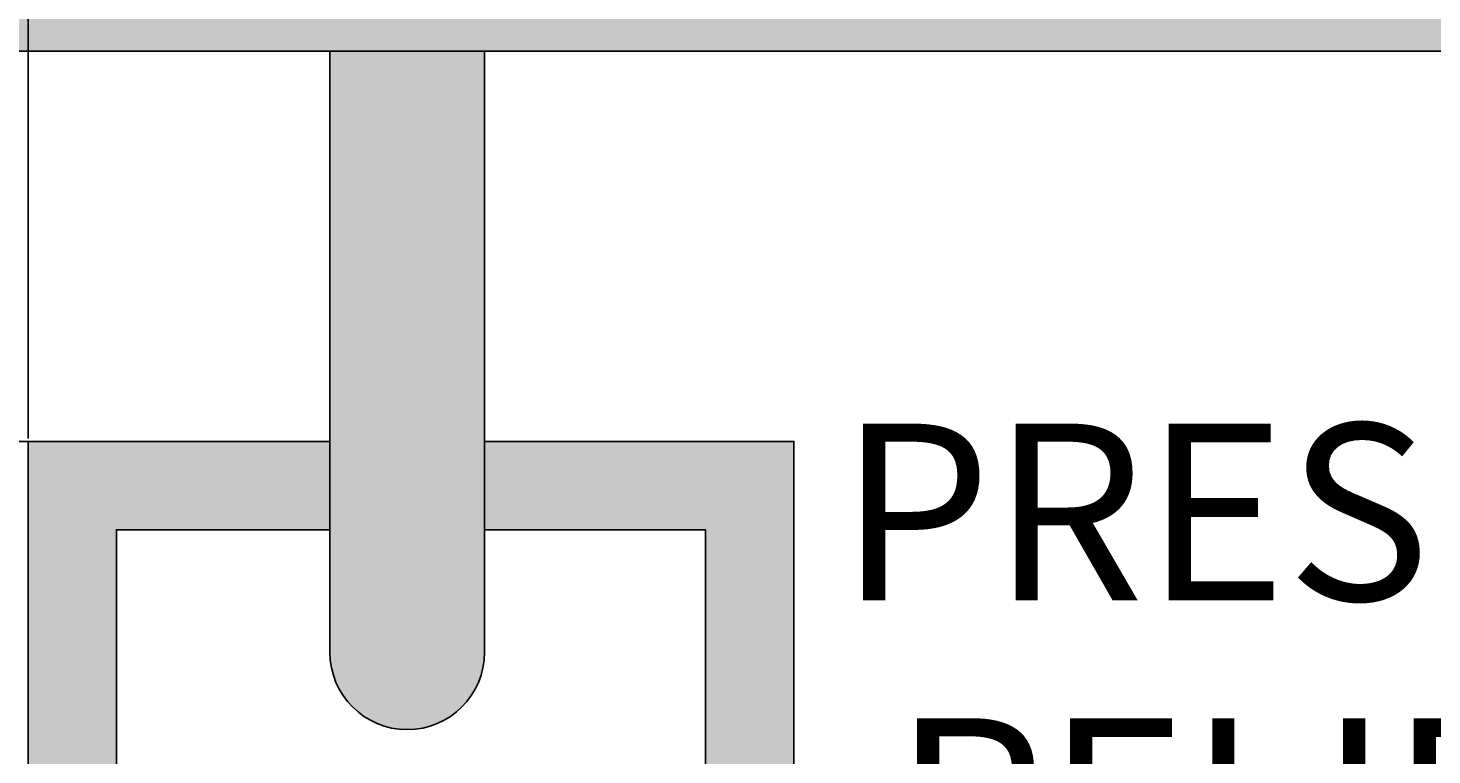
# Model space of a CAD drawing. Units: millimetres. Extents: x -11 to 280, y -4 to 208.
# Tile 24 of 55: x 119 to 150, y 89 to 106. Entities that reach past the tile are written whole.
import ezdxf

# ---------------------------------------------------------------- set-up
doc = ezdxf.new("R2010")
doc.units = ezdxf.units.MM
for name, color, linetype, lineweight in [('M-ANNO-TEXT', 7, 'Continuous', 18), ('M-DIMS', 2, 'Continuous', 18), ('M-HYDR-PRES', 7, 'Continuous', 25), ('M-HYDR-VALV', 7, 'Continuous', 25), ('M-HYDR-VALV-PATT', 252, 'Continuous', 13)]:
    doc.layers.add(name, color=color, linetype=linetype, lineweight=lineweight)
doc.layers.add('M-HYDR-PRES-PATT', color=240, linetype='Continuous', lineweight=13, true_color=0xed1f24)
doc.styles.get("Standard").update_dxf_attribs({"font": 'arial.ttf'})
doc.dimstyles.get("Standard").update_dxf_attribs({"dimtxt": 0.18, "dimasz": 0.18, "dimexe": 0.18, "dimexo": 0.0625, "dimgap": 0.09, "dimtad": 0, "dimtih": 1, "dimtoh": 1, "dimdec": 4, "dimzin": 0, "dimdsep": 46, "dimtxsty": 'Standard', "dimcen": 0.09, "dimadec": 0, "dimazin": 0, "dimtfac": 1, "dimtdec": 4, "dimtofl": 0, "dimtmove": 0, "dimatfit": 3, "dimfxl": 1, "dimtolj": 1, "dimtzin": 0, "dimarcsym": 0})

# ---------------------------------------------------------------- blocks, each defined once
blk = doc.blocks.new('*D5')
at = {"layer": 'Defpoints', "color": 0, "transparency": 16777216}
for p in [(24.759, 192.645), (-10.087, 11.435), (261.686, 11.435)]:
    blk.add_point(p, dxfattribs=at)
at = {"layer": 'M-DIMS', "color": 0, "lineweight": -2, "transparency": 16777216}
for p, q in [((24.696, 192.645), (-10.267, 192.645)), ((-10.087, 192.465), (-10.087, 102.222)), ((-10.087, 11.615), (-10.087, 101.858)), ((261.624, 11.435), (-10.267, 11.435))]:
    blk.add_line(p, q, dxfattribs=at)
at = {"layer": 'M-DIMS', "color": 0, "transparency": 16777216}
for points in [[(-10.117, 192.465), (-10.057, 192.465), (-10.087, 192.645)], [(-10.117, 11.615), (-10.057, 11.615), (-10.087, 11.435)]]:
    blk.add_solid(points, dxfattribs=at)
at = {"layer": 'M-DIMS', "color": 0, "transparency": 16777216, "insert": (-10.087, 102.04), "char_height": 0.18, "attachment_point": 5}
blk.add_mtext('\\A1;181.2', dxfattribs=at)
blk = doc.blocks.new('*D12')
at = {"layer": 'Defpoints', "color": 0, "transparency": 16777216}
for p in [(173.804, 207.495), (118.514, 96.485), (173.804, 89.387)]:
    blk.add_point(p, dxfattribs=at)
at = {"layer": 'M-DIMS', "color": 0, "lineweight": -2, "transparency": 16777216}
for p, q in [((118.514, 96.547), (118.514, 207.675)), ((118.694, 207.495), (145.765, 207.495)), ((173.624, 207.495), (146.553, 207.495)), ((173.804, 89.45), (173.804, 207.675))]:
    blk.add_line(p, q, dxfattribs=at)
at = {"layer": 'M-DIMS', "color": 0, "transparency": 16777216}
for points in [[(118.694, 207.525), (118.694, 207.465), (118.514, 207.495)], [(173.624, 207.525), (173.624, 207.465), (173.804, 207.495)]]:
    blk.add_solid(points, dxfattribs=at)
at = {"layer": 'M-DIMS', "color": 0, "transparency": 16777216, "insert": (146.159, 207.495), "char_height": 0.18, "attachment_point": 5}
blk.add_mtext('\\A1;55.29', dxfattribs=at)
blk = doc.blocks.new('*D16')
at = {"layer": 'Defpoints', "color": 0, "transparency": 16777216}
for p in [(110.493, 105.314), (125.343, 105.314), (125.343, 96.485)]:
    blk.add_point(p, dxfattribs=at)
at = {"layer": 'M-DIMS', "color": 0, "lineweight": -2, "transparency": 16777216}
for p, q in [((125.281, 105.314), (110.313, 105.314)), ((110.493, 105.134), (110.493, 101.081)), ((110.493, 96.665), (110.493, 100.718)), ((125.281, 96.485), (110.313, 96.485))]:
    blk.add_line(p, q, dxfattribs=at)
at = {"layer": 'M-DIMS', "color": 0, "transparency": 16777216}
for points in [[(110.463, 105.134), (110.523, 105.134), (110.493, 105.314)], [(110.463, 96.665), (110.523, 96.665), (110.493, 96.485)]]:
    blk.add_solid(points, dxfattribs=at)
at = {"layer": 'M-DIMS', "color": 0, "transparency": 16777216, "insert": (110.493, 100.9), "char_height": 0.18, "attachment_point": 5}
blk.add_mtext('\\A1;8.83', dxfattribs=at)

msp = doc.modelspace()

# ---------------------------------------------------------------- hatches: boundary and pattern name
at = {"layer": 'M-HYDR-PRES-PATT'}
h = msp.add_hatch(color=256, dxfattribs=at)
h.set_gradient(color1=(237, 31, 36), color2=(237, 31, 36), tint=1)
h.paths.add_polyline_path([(232.2, 133.1228), (228.7, 133.1228), (228.7, 108.8141), (102.7646, 108.8141), (102.7646, 105.3141), (232.2, 105.3141)])
h.paths.add_polyline_path([(128.8433, 105.3141), (125.3433, 105.3141), (125.3433, 91.7099, 1), (128.8433, 91.7099)])
h.paths.add_polyline_path([(229.1617, 78.7098), (196.7745, 78.7098, -0.4142136), (191.7745, 83.7098), (191.7745, 105.3141), (188.2745, 105.3141), (188.2745, 80.2098, 0.4142136), (193.2745, 75.2098), (225.6617, 75.2098), (225.6617, 43.5991), (229.1617, 43.5991)])
h.paths.add_polyline_path([(102.7646, 110.3704), (95.5776, 110.3704), (95.5776, 103.9022), (102.7646, 103.9022)])
h.paths.add_polyline_path([(100.7059, 107.2502), (99.1711, 106.3641), (99.1711, 106.8641), (97.1711, 106.8641), (97.1711, 107.6363), (99.1711, 107.6363), (99.1711, 108.1363)], flags=16)
h.paths.add_polyline_path([(234.6119, 138.4081), (226.5106, 138.4081), (226.5106, 133.1228), (234.6119, 133.1228)])
h.paths.add_polyline_path([(231.1963, 135.7055), (230.2965, 134.1786), (229.4241, 135.7213), (229.9241, 135.7168), (229.9418, 137.7167), (230.7141, 137.7099), (230.6963, 135.71)], flags=16)
at = {"layer": 'M-HYDR-VALV-PATT'}
h = msp.add_hatch(color=256, dxfattribs=at)
h.set_gradient(color1=(153, 153, 0), color2=(153, 153, 0), tint=1)
h.paths.add_polyline_path([(135.8437, 96.4849), (128.8433, 96.4849), (128.8433, 94.4849), (133.8437, 94.4849), (133.8437, 68.8227), (128.2568, 68.8227), (128.2568, 66.8227), (135.8437, 66.8227)])
h.paths.add_polyline_path([(126.2568, 68.8227), (120.5137, 68.8227), (120.5137, 70.8991), (118.5137, 70.8991), (118.5137, 66.8227), (126.2568, 66.8227)])
h.paths.add_polyline_path([(120.5137, 94.4849), (125.3433, 94.4849), (125.3433, 96.4849), (118.5137, 96.4849), (118.5137, 74.3991), (120.5137, 74.3991)])
h.paths.add_polyline_path([(128.2568, 72.69), (126.2568, 72.69), (126.2568, 64.0664), (128.2568, 64.0664)])
h.paths.add_polyline_path([(131.6327, 64.0664), (122.8484, 64.0664), (122.8484, 61.5587), (131.6327, 61.5587)])
h.paths.add_polyline_path([(133.8437, 73.5419), (120.5137, 73.5419), (120.5137, 72.69), (133.8437, 72.69)])

# ---------------------------------------------------------------- linework, layer by layer
at = {"layer": 'M-HYDR-PRES'}
for p, q in [((125.3433, 105.3141), (125.3433, 91.7099)), ((128.8433, 105.3141), (128.8433, 91.7099))]:
    msp.add_line(p, q, dxfattribs=at)
msp.add_lwpolyline([(232.2, 133.1228), (232.2, 105.3141), (102.7646, 105.3141)], dxfattribs=at)
msp.add_arc((127.0933, 91.7099), 1.75, 180, 0, dxfattribs=at)
at = {"layer": 'M-HYDR-VALV'}
for points in [[(118.5137, 74.3991), (118.5137, 96.4849), (125.3433, 96.4849)], [(128.8433, 96.4849), (135.8437, 96.4849), (135.8437, 66.8227), (128.2568, 66.8227)], [(126.2568, 68.8227), (120.5137, 68.8227), (120.5137, 94.4849), (125.3433, 94.4849)], [(128.8433, 94.4849), (133.8437, 94.4849), (133.8437, 68.8227), (128.2568, 68.8227)]]:
    msp.add_lwpolyline(points, dxfattribs=at)

# ---------------------------------------------------------------- texts
at = {"layer": 'M-ANNO-TEXT', "insert": (136.8574, 96.8862), "char_height": 4, "attachment_point": 1}
msp.add_mtext_dynamic_manual_height_columns('PRESSURE\\P RELIEF\\PVALVE', width=63.617875, gutter_width=12.5, heights=[0], dxfattribs=at)

# ---------------------------------------------------------------- dimensions: what is measured, and where the dimension line sits
at = {"layer": 'M-DIMS'}
dim = msp.add_linear_dim(base=(173.8038, 207.495), p1=(118.5137, 96.4849), p2=(173.8038, 89.3873), dimstyle='Standard', override={"dimdec": 2, "dimlfac": 1, "dimrnd": 0, "dimzin": 0, "dimdsep": 46, "dimlunit": 2}, dxfattribs=at)
dim.commit()
dim.dimension.update_dxf_attribs({"geometry": '*D12', "text_midpoint": (146.1587, 207.495)})
for base, p1, p2, override, picture, middle in [((-10.0865, 11.4346), (24.7588, 192.645), (261.6863, 11.4346), {"dimdec": 1, "dimlfac": 1, "dimrnd": 0, "dimzin": 0, "dimdsep": 46, "dimlunit": 2}, '*D5', (-10.0865, 102.0398)), ((110.4933, 105.3141), (125.3433, 96.4849), (125.3433, 105.3141), {"dimdec": 2, "dimlfac": 1, "dimrnd": 0, "dimzin": 0, "dimdsep": 46, "dimlunit": 2}, '*D16', (110.4933, 100.8995))]:
    dim = msp.add_linear_dim(base=base, p1=p1, p2=p2, angle=90, dimstyle='Standard', override=override, dxfattribs=at)
    dim.commit()
    dim.dimension.update_dxf_attribs({"geometry": picture, "text_midpoint": middle})

doc.saveas('drawing.dxf')
